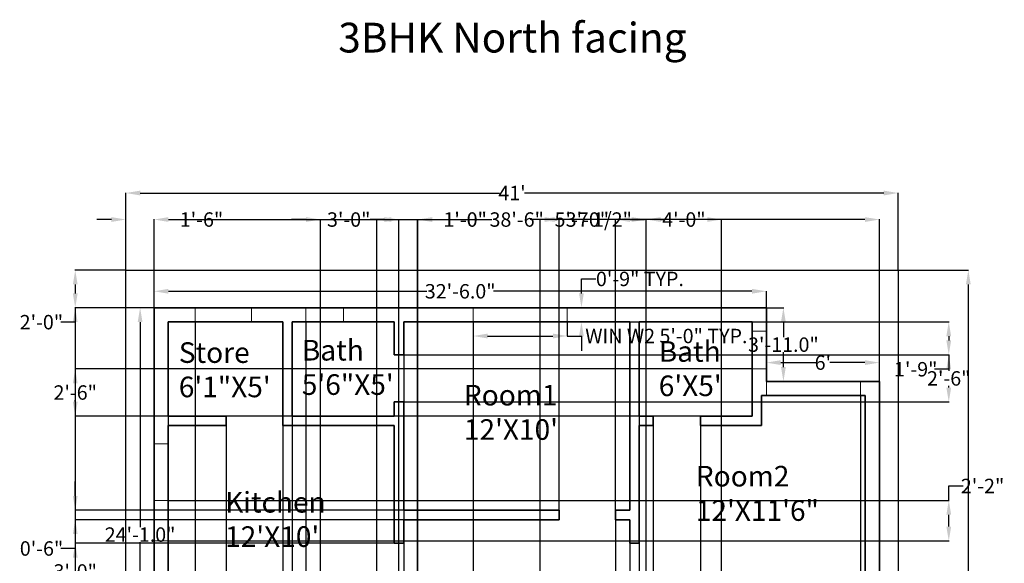
# Model space of a CAD drawing. Units: inches. Extents: x -69 to 558, y -494 to 191.
# Tile 3 of 3: x -69 to 558, y -155 to 191. Entities that reach past the tile are written whole.
import ezdxf

# ---------------------------------------------------------------- set-up
doc = ezdxf.new("R2010")
doc.units = ezdxf.units.IN
doc.header["$MEASUREMENT"] = 0
for name, color, linetype, lineweight in [('A-ANNO-DIMS', 2, 'Continuous', 18), ('A-ANNO-TEXT', 7, 'Continuous', 25), ('A-AREA-IDEN', 7, 'Continuous', 18), ('A-GLAZ', 4, 'Continuous', 18), ('A-WALL', 7, 'Continuous', 35), ('C-PROP', 8, 'Continuous', 25)]:
    doc.layers.add(name, color=color, linetype=linetype, lineweight=lineweight)
doc.styles.get("Standard").update_dxf_attribs({"font": 'arial.ttf'})
doc.dimstyles.get("Standard").update_dxf_attribs({"dimtxt": 9.18, "dimasz": 9.18, "dimexe": 0.18, "dimexo": 0.0625, "dimgap": 0.09, "dimtad": 0, "dimtih": 1, "dimtoh": 1, "dimdec": 1, "dimzin": 0, "dimdsep": 46, "dimlunit": 3, "dimtxsty": 'Standard', "dimcen": 9, "dimadec": 0, "dimazin": 0, "dimtfac": 1, "dimtdec": 1, "dimtofl": 0, "dimtmove": 0, "dimatfit": 3, "dimfxl": 1, "dimtolj": 1, "dimtzin": 0, "dimarcsym": 0})

# ---------------------------------------------------------------- blocks, each defined once
blk = doc.blocks.new('*D8')
at = {"layer": 'A-ANNO-DIMS', "color": 0, "lineweight": -2, "transparency": 16777216}
for p, q in [((490.42, 31.7), (535.2, 31.7)), ((535.02, 22.52), (535.02, -203.53)), ((535.02, -439.12), (535.02, -213.08)), ((490.42, -448.3), (535.2, -448.3))]:
    blk.add_line(p, q, dxfattribs=at)
at = {"layer": 'A-ANNO-DIMS', "color": 0, "transparency": 16777216}
for points in [[(533.49, 22.52), (536.55, 22.52), (535.02, 31.7)], [(533.49, -439.12), (536.55, -439.12), (535.02, -448.3)]]:
    blk.add_solid(points, dxfattribs=at)
at = {"layer": 'Defpoints', "color": 0, "transparency": 16777216}
for p in [(490.36, 31.7), (490.36, -448.3), (535.02, -448.3)]:
    blk.add_point(p, dxfattribs=at)
at = {"layer": 'A-ANNO-DIMS', "color": 0, "transparency": 16777216, "insert": (535.02, -208.3), "char_height": 9.18, "attachment_point": 5}
blk.add_mtext("\\A1;40'", dxfattribs=at)
blk = doc.blocks.new('*D9')
at = {"layer": 'A-ANNO-DIMS', "color": 0, "lineweight": -2, "transparency": 16777216}
for p, q in [((-1.64, 31.76), (-1.64, 80.97)), ((7.54, 80.79), (236.29, 80.79)), ((481.18, 80.79), (252.42, 80.79)), ((490.36, 31.76), (490.36, 80.97))]:
    blk.add_line(p, q, dxfattribs=at)
at = {"layer": 'A-ANNO-DIMS', "color": 0, "transparency": 16777216}
for points in [[(7.54, 82.32), (7.54, 79.26), (-1.64, 80.79)], [(481.18, 82.32), (481.18, 79.26), (490.36, 80.79)]]:
    blk.add_solid(points, dxfattribs=at)
at = {"layer": 'Defpoints', "color": 0, "transparency": 16777216}
for p in [(490.36, 80.79), (-1.64, 31.7), (490.36, 31.7)]:
    blk.add_point(p, dxfattribs=at)
at = {"layer": 'A-ANNO-DIMS', "color": 0, "transparency": 16777216, "insert": (244.36, 80.79), "char_height": 9.18, "attachment_point": 5}
blk.add_mtext("\\A1;41'", dxfattribs=at)
blk = doc.blocks.new('*D10')
at = {"layer": 'A-ANNO-DIMS', "color": 0, "lineweight": -2, "transparency": 16777216}
for p, q in [((16.36, 7.76), (16.36, 18.37)), ((25.54, 18.19), (190.16, 18.19)), ((397.18, 18.19), (232.56, 18.19)), ((406.36, 7.76), (406.36, 18.37))]:
    blk.add_line(p, q, dxfattribs=at)
at = {"layer": 'A-ANNO-DIMS', "color": 0, "transparency": 16777216}
for points in [[(25.54, 19.72), (25.54, 16.66), (16.36, 18.19)], [(397.18, 19.72), (397.18, 16.66), (406.36, 18.19)]]:
    blk.add_solid(points, dxfattribs=at)
at = {"layer": 'Defpoints', "color": 0, "transparency": 16777216}
for p in [(406.36, 18.19), (16.36, 7.7), (406.36, 7.7)]:
    blk.add_point(p, dxfattribs=at)
at = {"layer": 'A-ANNO-DIMS', "color": 0, "transparency": 16777216, "insert": (211.36, 18.19), "char_height": 9.18, "attachment_point": 5}
blk.add_mtext('\\A1;32\'-6.0"', dxfattribs=at)
blk = doc.blocks.new('*D11')
at = {"layer": 'A-ANNO-DIMS', "color": 0, "lineweight": -2, "transparency": 16777216}
for p, q in [((406.36, -39.24), (406.36, -27.06)), ((415.54, -27.24), (438.02, -27.24)), ((469.18, -27.24), (446.7, -27.24)), ((478.36, -39.24), (478.36, -27.06))]:
    blk.add_line(p, q, dxfattribs=at)
at = {"layer": 'A-ANNO-DIMS', "color": 0, "transparency": 16777216}
for points in [[(415.54, -25.71), (415.54, -28.77), (406.36, -27.24)], [(469.18, -25.71), (469.18, -28.77), (478.36, -27.24)]]:
    blk.add_solid(points, dxfattribs=at)
at = {"layer": 'Defpoints', "color": 0, "transparency": 16777216}
for p in [(478.36, -27.24), (406.36, -39.3), (478.36, -39.3)]:
    blk.add_point(p, dxfattribs=at)
at = {"layer": 'A-ANNO-DIMS', "color": 0, "transparency": 16777216, "insert": (442.36, -27.24), "char_height": 9.18, "attachment_point": 5}
blk.add_mtext("\\A1;6'", dxfattribs=at)
blk = doc.blocks.new('*D12')
at = {"layer": 'A-ANNO-DIMS', "color": 0, "lineweight": -2, "transparency": 16777216}
for p, q in [((406.42, 7.7), (417.41, 7.7)), ((417.23, -1.48), (417.23, -11.02)), ((417.23, -30.12), (417.23, -20.59)), ((406.42, -39.3), (417.41, -39.3))]:
    blk.add_line(p, q, dxfattribs=at)
at = {"layer": 'A-ANNO-DIMS', "color": 0, "transparency": 16777216}
for points in [[(415.7, -1.48), (418.76, -1.48), (417.23, 7.7)], [(415.7, -30.12), (418.76, -30.12), (417.23, -39.3)]]:
    blk.add_solid(points, dxfattribs=at)
at = {"layer": 'Defpoints', "color": 0, "transparency": 16777216}
for p in [(406.36, 7.7), (417.23, 7.7), (406.36, -39.3)]:
    blk.add_point(p, dxfattribs=at)
at = {"layer": 'A-ANNO-DIMS', "color": 0, "transparency": 16777216, "insert": (417.23, -15.8), "char_height": 9.18, "attachment_point": 5}
blk.add_mtext('\\A1;3\'-11.0"', dxfattribs=at)
blk = doc.blocks.new('*D13')
at = {"layer": 'A-ANNO-DIMS', "color": 0, "lineweight": -2, "transparency": 16777216}
for p, q in [((16.29, 7.7), (7.29, 7.7)), ((7.47, -1.48), (7.47, -132.03)), ((7.47, -272.12), (7.47, -141.58)), ((16.29, -281.3), (7.29, -281.3))]:
    blk.add_line(p, q, dxfattribs=at)
at = {"layer": 'A-ANNO-DIMS', "color": 0, "transparency": 16777216}
for points in [[(5.94, -1.48), (9, -1.48), (7.47, 7.7)], [(5.94, -272.12), (9, -272.12), (7.47, -281.3)]]:
    blk.add_solid(points, dxfattribs=at)
at = {"layer": 'Defpoints', "color": 0, "transparency": 16777216}
for p in [(7.47, 7.7), (16.36, 7.7), (16.36, -281.3)]:
    blk.add_point(p, dxfattribs=at)
at = {"layer": 'A-ANNO-DIMS', "color": 0, "transparency": 16777216, "insert": (7.47, -136.8), "char_height": 9.18, "attachment_point": 5}
blk.add_mtext('\\A1;24\'-1.0"', dxfattribs=at)
blk = doc.blocks.new('WIN-36IN')
blk.add_lwpolyline([(0, 0), (0, 9), (36, 9), (36, 0)], close=True)
blk = doc.blocks.new('WIN-60IN')
blk.add_lwpolyline([(60, 9), (60, 0), (0, 0), (0, 9)], close=True)
blk = doc.blocks.new('WIN-24IN')
blk.add_lwpolyline([(0, 0), (0, 9), (24, 9), (24, 0)], close=True)
blk = doc.blocks.new('*D20')
at = {"layer": 'A-ANNO-DIMS', "color": 0, "lineweight": -2, "transparency": 16777216}
for p, q in [((219.59, -1.37), (219.59, -10.48)), ((279.59, -1.37), (279.59, -10.48)), ((228.77, -10.3), (270.41, -10.3)), ((279.59, -10.3), (288.77, -10.3))]:
    blk.add_line(p, q, dxfattribs=at)
at = {"layer": 'A-ANNO-DIMS', "color": 0, "transparency": 16777216}
for points in [[(228.77, -8.77), (228.77, -11.83), (219.59, -10.3)], [(270.41, -8.77), (270.41, -11.83), (279.59, -10.3)]]:
    blk.add_solid(points, dxfattribs=at)
at = {"layer": 'Defpoints', "color": 0, "transparency": 16777216}
for p in [(219.59, -1.3), (279.59, -1.3), (279.59, -10.3)]:
    blk.add_point(p, dxfattribs=at)
at = {"layer": 'A-ANNO-DIMS', "color": 0, "transparency": 16777216, "insert": (342.67, -10.3), "char_height": 9.18, "attachment_point": 5}
blk.add_mtext('\\A1;WIN W2 5\'-0" TYP.', dxfattribs=at)
blk = doc.blocks.new('*D21')
at = {"layer": 'A-ANNO-DIMS', "color": 0, "lineweight": -2, "transparency": 16777216}
for p, q in [((288.59, 16.88), (288.59, 26.06)), ((288.59, 26.06), (297.77, 26.06)), ((279.66, 7.7), (288.77, 7.7)), ((279.66, -1.3), (288.77, -1.3)), ((288.59, -10.48), (288.59, -19.66))]:
    blk.add_line(p, q, dxfattribs=at)
at = {"layer": 'A-ANNO-DIMS', "color": 0, "transparency": 16777216}
for points in [[(287.06, 16.88), (290.12, 16.88), (288.59, 7.7)], [(287.06, -10.48), (290.12, -10.48), (288.59, -1.3)]]:
    blk.add_solid(points, dxfattribs=at)
at = {"layer": 'Defpoints', "color": 0, "transparency": 16777216}
for p in [(279.59, 7.7), (288.59, 7.7), (279.59, -1.3)]:
    blk.add_point(p, dxfattribs=at)
at = {"layer": 'A-ANNO-DIMS', "color": 0, "transparency": 16777216, "insert": (325.84, 26.06), "char_height": 9.18, "attachment_point": 5}
blk.add_mtext('\\A1;0\'-9" TYP.', dxfattribs=at)
blk = doc.blocks.new('*D24')
at = {"layer": 'A-ANNO-DIMS', "color": 0, "lineweight": -2, "transparency": 16777216}
for p, q in [((16.36, 7.76), (16.36, 64.08)), ((25.54, 63.9), (231.5, 63.9)), ((469.18, 63.9), (263.21, 63.9)), ((478.36, -39.24), (478.36, 64.08))]:
    blk.add_line(p, q, dxfattribs=at)
at = {"layer": 'A-ANNO-DIMS', "color": 0, "transparency": 16777216}
for points in [[(25.54, 65.43), (25.54, 62.37), (16.36, 63.9)], [(469.18, 65.43), (469.18, 62.37), (478.36, 63.9)]]:
    blk.add_solid(points, dxfattribs=at)
at = {"layer": 'Defpoints', "color": 0, "transparency": 16777216}
for p in [(478.36, 63.9), (16.36, 7.7), (478.36, -39.3)]:
    blk.add_point(p, dxfattribs=at)
at = {"layer": 'A-ANNO-DIMS', "color": 0, "transparency": 16777216, "insert": (247.36, 63.9), "char_height": 9.18, "attachment_point": 5}
blk.add_mtext('\\A1;38\'-6"', dxfattribs=at)
blk = doc.blocks.new('*D25')
at = {"layer": 'A-ANNO-DIMS', "color": 0, "lineweight": -2, "transparency": 16777216}
for p, q in [((16.29, 7.7), (-34.02, 7.7)), ((-33.84, -1.48), (-33.84, -203.52)), ((-33.84, -415.12), (-33.84, -213.09)), ((172.29, -424.3), (-34.02, -424.3))]:
    blk.add_line(p, q, dxfattribs=at)
at = {"layer": 'A-ANNO-DIMS', "color": 0, "transparency": 16777216}
for points in [[(-35.37, -1.48), (-32.31, -1.48), (-33.84, 7.7)], [(-35.37, -415.12), (-32.31, -415.12), (-33.84, -424.3)]]:
    blk.add_solid(points, dxfattribs=at)
at = {"layer": 'Defpoints', "color": 0, "transparency": 16777216}
for p in [(16.36, 7.7), (-33.84, -424.3), (172.36, -424.3)]:
    blk.add_point(p, dxfattribs=at)
at = {"layer": 'A-ANNO-DIMS', "color": 0, "transparency": 16777216, "insert": (-33.84, -208.3), "char_height": 9.18, "attachment_point": 5}
blk.add_mtext('\\A1;36\'-0"', dxfattribs=at)
blk = doc.blocks.new('*D26')
at = {"layer": 'A-ANNO-DIMS', "color": 0, "lineweight": -2, "transparency": 16777216}
for p, q in [((-10.82, 63.9), (-20, 63.9)), ((-1.64, 31.76), (-1.64, 64.08)), ((16.36, 7.76), (16.36, 64.08)), ((25.54, 63.9), (34.72, 63.9))]:
    blk.add_line(p, q, dxfattribs=at)
at = {"layer": 'A-ANNO-DIMS', "color": 0, "transparency": 16777216}
for points in [[(-10.82, 65.43), (-10.82, 62.37), (-1.64, 63.9)], [(25.54, 65.43), (25.54, 62.37), (16.36, 63.9)]]:
    blk.add_solid(points, dxfattribs=at)
at = {"layer": 'Defpoints', "color": 0, "transparency": 16777216}
for p in [(16.36, 63.9), (-1.64, 31.7), (16.36, 7.7)]:
    blk.add_point(p, dxfattribs=at)
at = {"layer": 'A-ANNO-DIMS', "color": 0, "transparency": 16777216, "insert": (46.58, 63.9), "char_height": 9.18, "attachment_point": 5}
blk.add_mtext('\\A1;1\'-6"', dxfattribs=at)
blk = doc.blocks.new('*D27')
at = {"layer": 'A-ANNO-DIMS', "color": 0, "lineweight": -2, "transparency": 16777216}
for p, q in [((-1.71, 31.7), (-34.02, 31.7)), ((-33.84, 22.52), (-33.84, 16.88)), ((16.29, 7.7), (-34.02, 7.7)), ((-33.84, 7.7), (-33.84, -1.48)), ((-33.84, -1.48), (-43.02, -1.48))]:
    blk.add_line(p, q, dxfattribs=at)
at = {"layer": 'A-ANNO-DIMS', "color": 0, "transparency": 16777216}
for points in [[(-35.37, 22.52), (-32.31, 22.52), (-33.84, 31.7)], [(-35.37, 16.88), (-32.31, 16.88), (-33.84, 7.7)]]:
    blk.add_solid(points, dxfattribs=at)
at = {"layer": 'Defpoints', "color": 0, "transparency": 16777216}
for p in [(-1.64, 31.7), (-33.84, 7.7), (16.36, 7.7)]:
    blk.add_point(p, dxfattribs=at)
at = {"layer": 'A-ANNO-DIMS', "color": 0, "transparency": 16777216, "insert": (-55.39, -1.48), "char_height": 9.18, "attachment_point": 5}
blk.add_mtext('\\A1;2\'-0"', dxfattribs=at)
blk = doc.blocks.new('*D30')
at = {"layer": 'A-ANNO-DIMS', "color": 0, "lineweight": -2, "transparency": 16777216}
for p, q in [((113.177437, 63.89515), (103.997437, 63.89515)), ((122.357437, -267.24235), (122.357437, 64.07515)), ((158.357437, -267.24235), (158.357437, 64.07515)), ((167.537437, 63.89515), (176.717437, 63.89515))]:
    blk.add_line(p, q, dxfattribs=at)
at = {"layer": 'A-ANNO-DIMS', "color": 0, "transparency": 16777216}
for points in [[(113.177437, 65.42515), (113.177437, 62.36515), (122.357437, 63.89515)], [(167.537437, 65.42515), (167.537437, 62.36515), (158.357437, 63.89515)]]:
    blk.add_solid(points, dxfattribs=at)
at = {"layer": 'Defpoints', "color": 0, "transparency": 16777216}
for p in [(158.357437, 63.89515), (122.357437, -267.30485), (158.357437, -267.30485)]:
    blk.add_point(p, dxfattribs=at)
at = {"layer": 'A-ANNO-DIMS', "color": 0, "transparency": 16777216, "insert": (140.357437, 63.89515), "char_height": 9.18, "attachment_point": 5}
blk.add_mtext('\\A1;3\'-0"', dxfattribs=at)
blk = doc.blocks.new('*D32')
at = {"layer": 'A-ANNO-DIMS', "color": 0, "lineweight": -2, "transparency": 16777216}
for p, q in [((163.09, 63.9), (153.91, 63.9)), ((172.27, -311.24), (172.27, 64.08)), ((184.27, -311.24), (184.27, 64.08)), ((193.45, 63.9), (202.63, 63.9))]:
    blk.add_line(p, q, dxfattribs=at)
at = {"layer": 'A-ANNO-DIMS', "color": 0, "transparency": 16777216}
for points in [[(163.09, 65.43), (163.09, 62.37), (172.27, 63.9)], [(193.45, 65.43), (193.45, 62.37), (184.27, 63.9)]]:
    blk.add_solid(points, dxfattribs=at)
at = {"layer": 'Defpoints', "color": 0, "transparency": 16777216}
for p in [(184.27, 63.9), (172.27, -311.3), (184.27, -311.3)]:
    blk.add_point(p, dxfattribs=at)
at = {"layer": 'A-ANNO-DIMS', "color": 0, "transparency": 16777216, "insert": (214.49, 63.9), "char_height": 9.18, "attachment_point": 5}
blk.add_mtext('\\A1;1\'-0"', dxfattribs=at)
blk = doc.blocks.new('*D33')
at = {"layer": 'A-ANNO-DIMS', "color": 0, "lineweight": -2, "transparency": 16777216}
for p, q in [((329.86, -415.24), (329.86, 64.08)), ((339.04, 63.9), (341.38, 63.9)), ((368.68, 63.9), (366.33, 63.9)), ((377.86, -415.24), (377.86, 64.08))]:
    blk.add_line(p, q, dxfattribs=at)
at = {"layer": 'A-ANNO-DIMS', "color": 0, "transparency": 16777216}
for points in [[(339.04, 65.43), (339.04, 62.37), (329.86, 63.9)], [(368.68, 65.43), (368.68, 62.37), (377.86, 63.9)]]:
    blk.add_solid(points, dxfattribs=at)
at = {"layer": 'Defpoints', "color": 0, "transparency": 16777216}
for p in [(377.86, 63.9), (329.86, -415.3), (377.86, -415.3)]:
    blk.add_point(p, dxfattribs=at)
at = {"layer": 'A-ANNO-DIMS', "color": 0, "transparency": 16777216, "insert": (353.86, 63.9), "char_height": 9.18, "attachment_point": 5}
blk.add_mtext('\\A1;4\'-0"', dxfattribs=at)
blk = doc.blocks.new('*D34')
at = {"layer": 'A-ANNO-DIMS', "color": 0, "lineweight": -2, "transparency": 16777216}
for p, q in [((265.177437, 63.89515), (255.997437, 63.89515)), ((274.357437, -121.24235), (274.357437, 64.07515)), ((310.357437, -121.24235), (310.357437, 64.07515)), ((319.537437, 63.89515), (328.717437, 63.89515))]:
    blk.add_line(p, q, dxfattribs=at)
at = {"layer": 'A-ANNO-DIMS', "color": 0, "transparency": 16777216}
for points in [[(265.177437, 65.42515), (265.177437, 62.36515), (274.357437, 63.89515)], [(319.537437, 65.42515), (319.537437, 62.36515), (310.357437, 63.89515)]]:
    blk.add_solid(points, dxfattribs=at)
at = {"layer": 'Defpoints', "color": 0, "transparency": 16777216}
for p in [(310.357437, 63.89515), (274.357437, -121.30485), (310.357437, -121.30485)]:
    blk.add_point(p, dxfattribs=at)
at = {"layer": 'A-ANNO-DIMS', "color": 0, "transparency": 16777216, "insert": (292.357437, 63.89515), "char_height": 9.18, "attachment_point": 5}
blk.add_mtext('\\A1;3\'-0"', dxfattribs=at)
blk = doc.blocks.new('*D35')
at = {"layer": 'A-ANNO-DIMS', "color": 0, "lineweight": -2, "transparency": 16777216}
for p, q in [((334.357437, -67.36735), (334.357437, -480.68485)), ((364.357437, -67.36735), (364.357437, -480.68485)), ((325.177437, -480.50485), (315.997437, -480.50485)), ((373.537437, -480.50485), (382.717437, -480.50485))]:
    blk.add_line(p, q, dxfattribs=at)
at = {"layer": 'A-ANNO-DIMS', "color": 0, "transparency": 16777216}
for points in [[(325.177437, -478.97485), (325.177437, -482.03485), (334.357437, -480.50485)], [(373.537437, -478.97485), (373.537437, -482.03485), (364.357437, -480.50485)]]:
    blk.add_solid(points, dxfattribs=at)
at = {"layer": 'Defpoints', "color": 0, "transparency": 16777216}
for p in [(334.357437, -67.30485), (364.357437, -67.30485), (364.357437, -480.50485)]:
    blk.add_point(p, dxfattribs=at)
at = {"layer": 'A-ANNO-DIMS', "color": 0, "transparency": 16777216, "insert": (349.357437, -480.50485), "char_height": 9.18, "attachment_point": 5}
blk.add_mtext('\\A1;2\'-6"', dxfattribs=at)
blk = doc.blocks.new('*D36')
at = {"layer": 'A-ANNO-DIMS', "color": 0, "lineweight": -2, "transparency": 16777216}
for p, q in [((-33.84, -112.12), (-33.84, -102.94)), ((274.29, -121.3), (-34.02, -121.3)), ((274.29, -127.3), (-34.02, -127.3)), ((-33.84, -136.48), (-33.84, -145.66)), ((-33.84, -145.66), (-43.02, -145.66))]:
    blk.add_line(p, q, dxfattribs=at)
at = {"layer": 'A-ANNO-DIMS', "color": 0, "transparency": 16777216}
for points in [[(-35.37, -112.12), (-32.31, -112.12), (-33.84, -121.3)], [(-35.37, -136.48), (-32.31, -136.48), (-33.84, -127.3)]]:
    blk.add_solid(points, dxfattribs=at)
at = {"layer": 'Defpoints', "color": 0, "transparency": 16777216}
for p in [(274.36, -121.3), (-33.84, -127.3), (274.36, -127.3)]:
    blk.add_point(p, dxfattribs=at)
at = {"layer": 'A-ANNO-DIMS', "color": 0, "transparency": 16777216, "insert": (-55.31, -145.66), "char_height": 9.18, "attachment_point": 5}
blk.add_mtext('\\A1;0\'-6"', dxfattribs=at)
blk = doc.blocks.new('*D37')
at = {"layer": 'A-ANNO-DIMS', "color": 0, "lineweight": -2, "transparency": 16777216}
for p, q in [((175.36, -1.37), (175.36, -480.68)), ((219.59, -1.37), (219.59, -480.68)), ((184.54, -480.5), (185.19, -480.5)), ((210.41, -480.5), (209.76, -480.5))]:
    blk.add_line(p, q, dxfattribs=at)
at = {"layer": 'A-ANNO-DIMS', "color": 0, "transparency": 16777216}
for points in [[(184.54, -478.97), (184.54, -482.03), (175.36, -480.5)], [(210.41, -478.97), (210.41, -482.03), (219.59, -480.5)]]:
    blk.add_solid(points, dxfattribs=at)
at = {"layer": 'Defpoints', "color": 0, "transparency": 16777216}
for p in [(175.36, -1.3), (219.59, -1.3), (219.59, -480.5)]:
    blk.add_point(p, dxfattribs=at)
at = {"layer": 'A-ANNO-DIMS', "color": 0, "transparency": 16777216, "insert": (197.48, -480.5), "char_height": 9.18, "attachment_point": 5}
blk.add_mtext('\\A1;3\'-8"', dxfattribs=at)
blk = doc.blocks.new('*D40')
at = {"layer": 'A-ANNO-DIMS', "color": 0, "lineweight": -2, "transparency": 16777216}
for p, q in [((25.36, -1.37), (25.36, -480.68)), ((42.48, -1.37), (42.48, -480.68)), ((16.18, -480.5), (7, -480.5)), ((51.66, -480.5), (60.84, -480.5))]:
    blk.add_line(p, q, dxfattribs=at)
at = {"layer": 'A-ANNO-DIMS', "color": 0, "transparency": 16777216}
for points in [[(16.18, -478.97), (16.18, -482.03), (25.36, -480.5)], [(51.66, -478.97), (51.66, -482.03), (42.48, -480.5)]]:
    blk.add_solid(points, dxfattribs=at)
at = {"layer": 'Defpoints', "color": 0, "transparency": 16777216}
for p in [(25.36, -1.3), (42.48, -1.3), (42.48, -480.5)]:
    blk.add_point(p, dxfattribs=at)
at = {"layer": 'A-ANNO-DIMS', "color": 0, "transparency": 16777216, "insert": (72.7, -480.5), "char_height": 9.18, "attachment_point": 5}
blk.add_mtext('\\A1;1\'-5"', dxfattribs=at)
blk = doc.blocks.new('*D41')
at = {"layer": 'A-ANNO-DIMS', "color": 0, "lineweight": -2, "transparency": 16777216}
for p, q in [((104.36, -1.37), (104.36, -480.68)), ((113.07, -1.37), (113.07, -480.68)), ((95.18, -480.5), (86, -480.5)), ((122.25, -480.5), (131.43, -480.5))]:
    blk.add_line(p, q, dxfattribs=at)
at = {"layer": 'A-ANNO-DIMS', "color": 0, "transparency": 16777216}
for points in [[(95.18, -478.97), (95.18, -482.03), (104.36, -480.5)], [(122.25, -478.97), (122.25, -482.03), (113.07, -480.5)]]:
    blk.add_solid(points, dxfattribs=at)
at = {"layer": 'Defpoints', "color": 0, "transparency": 16777216}
for p in [(104.36, -1.3), (113.07, -1.3), (113.07, -480.5)]:
    blk.add_point(p, dxfattribs=at)
at = {"layer": 'A-ANNO-DIMS', "color": 0, "transparency": 16777216, "insert": (154.42, -480.5), "char_height": 9.18, "attachment_point": 5}
blk.add_mtext('\\A1;0\'-8 1/2"', dxfattribs=at)
blk = doc.blocks.new('*D42')
at = {"layer": 'A-ANNO-DIMS', "color": 0, "lineweight": -2, "transparency": 16777216}
for p, q in [((397.29, -31.3), (-34.02, -31.3)), ((-33.84, -40.48), (-33.84, -41.53)), ((-33.84, -52.12), (-33.84, -51.08)), ((397.29, -61.3), (-34.02, -61.3))]:
    blk.add_line(p, q, dxfattribs=at)
at = {"layer": 'A-ANNO-DIMS', "color": 0, "transparency": 16777216}
for points in [[(-35.37, -40.48), (-32.31, -40.48), (-33.84, -31.3)], [(-35.37, -52.12), (-32.31, -52.12), (-33.84, -61.3)]]:
    blk.add_solid(points, dxfattribs=at)
at = {"layer": 'Defpoints', "color": 0, "transparency": 16777216}
for p in [(397.36, -31.3), (-33.84, -61.3), (397.36, -61.3)]:
    blk.add_point(p, dxfattribs=at)
at = {"layer": 'A-ANNO-DIMS', "color": 0, "transparency": 16777216, "insert": (-33.84, -46.3), "char_height": 9.18, "attachment_point": 5}
blk.add_mtext('\\A1;2\'-6"', dxfattribs=at)
blk = doc.blocks.new('*D43')
at = {"layer": 'A-ANNO-DIMS', "color": 0, "lineweight": -2, "transparency": 16777216}
for p, q in [((466.36, -48.37), (466.36, -480.68)), ((469.36, -48.37), (469.36, -480.68)), ((457.18, -480.5), (448, -480.5)), ((478.54, -480.5), (487.72, -480.5))]:
    blk.add_line(p, q, dxfattribs=at)
at = {"layer": 'A-ANNO-DIMS', "color": 0, "transparency": 16777216}
for points in [[(457.18, -478.97), (457.18, -482.03), (466.36, -480.5)], [(478.54, -478.97), (478.54, -482.03), (469.36, -480.5)]]:
    blk.add_solid(points, dxfattribs=at)
at = {"layer": 'Defpoints', "color": 0, "transparency": 16777216}
for p in [(466.36, -48.3), (469.36, -48.3), (469.36, -480.5)]:
    blk.add_point(p, dxfattribs=at)
at = {"layer": 'A-ANNO-DIMS', "color": 0, "transparency": 16777216, "insert": (500.01, -480.5), "char_height": 9.18, "attachment_point": 5}
blk.add_mtext('\\A1;0\'-3"', dxfattribs=at)
blk = doc.blocks.new('*D45')
at = {"layer": 'A-ANNO-DIMS', "color": 0, "lineweight": -2, "transparency": 16777216}
for p, q in [((522.56, -115.02), (522.56, -105.84)), ((522.56, -105.84), (531.74, -105.84)), ((25.42, -115.02), (522.74, -115.02)), ((522.56, -131.69), (522.56, -124.2)), ((25.42, -140.87), (522.74, -140.87))]:
    blk.add_line(p, q, dxfattribs=at)
at = {"layer": 'A-ANNO-DIMS', "color": 0, "transparency": 16777216}
for points in [[(521.03, -124.2), (524.09, -124.2), (522.56, -115.02)], [(521.03, -131.69), (524.09, -131.69), (522.56, -140.87)]]:
    blk.add_solid(points, dxfattribs=at)
at = {"layer": 'Defpoints', "color": 0, "transparency": 16777216}
for p in [(25.36, -115.02), (522.56, -115.02), (25.36, -140.87)]:
    blk.add_point(p, dxfattribs=at)
at = {"layer": 'A-ANNO-DIMS', "color": 0, "transparency": 16777216, "insert": (544.11, -105.84), "char_height": 9.18, "attachment_point": 5}
blk.add_mtext('\\A1;2\'-2"', dxfattribs=at)
blk = doc.blocks.new('*D47')
at = {"layer": 'A-ANNO-DIMS', "color": 0, "lineweight": -2, "transparency": 16777216}
for p, q in [((262.36, -415.24), (262.36, 64.08)), ((271.54, 63.9), (273.12, 63.9)), ((320.68, 63.9), (319.09, 63.9)), ((329.86, -415.24), (329.86, 64.08))]:
    blk.add_line(p, q, dxfattribs=at)
at = {"layer": 'A-ANNO-DIMS', "color": 0, "transparency": 16777216}
for points in [[(271.54, 65.43), (271.54, 62.37), (262.36, 63.9)], [(320.68, 65.43), (320.68, 62.37), (329.86, 63.9)]]:
    blk.add_solid(points, dxfattribs=at)
at = {"layer": 'Defpoints', "color": 0, "transparency": 16777216}
for p in [(329.86, 63.9), (262.36, -415.3), (329.86, -415.3)]:
    blk.add_point(p, dxfattribs=at)
at = {"layer": 'A-ANNO-DIMS', "color": 0, "transparency": 16777216, "insert": (296.11, 63.9), "char_height": 9.18, "attachment_point": 5}
blk.add_mtext('\\A1;5\'-7 1/2"', dxfattribs=at)
blk = doc.blocks.new('*D48')
at = {"layer": 'A-ANNO-DIMS', "color": 0, "lineweight": -2, "transparency": 16777216}
for p, q in [((310.36, -127.37), (310.36, -480.68)), ((319.36, -127.37), (319.36, -480.68)), ((301.18, -480.5), (292, -480.5)), ((328.54, -480.5), (337.72, -480.5))]:
    blk.add_line(p, q, dxfattribs=at)
at = {"layer": 'A-ANNO-DIMS', "color": 0, "transparency": 16777216}
for points in [[(301.18, -478.97), (301.18, -482.03), (310.36, -480.5)], [(328.54, -478.97), (328.54, -482.03), (319.36, -480.5)]]:
    blk.add_solid(points, dxfattribs=at)
at = {"layer": 'Defpoints', "color": 0, "transparency": 16777216}
for p in [(310.36, -127.3), (319.36, -127.3), (319.36, -480.5)]:
    blk.add_point(p, dxfattribs=at)
at = {"layer": 'A-ANNO-DIMS', "color": 0, "transparency": 16777216, "insert": (350.01, -480.5), "char_height": 9.18, "attachment_point": 5}
blk.add_mtext('\\A1;0\'-9"', dxfattribs=at)
blk = doc.blocks.new('*D49')
at = {"layer": 'A-ANNO-DIMS', "color": 0, "lineweight": -2, "transparency": 16777216}
for p, q in [((325.36, -61.37), (325.36, -480.68)), ((334.36, -61.37), (334.36, -480.68)), ((316.18, -480.5), (307, -480.5)), ((343.54, -480.5), (352.72, -480.5))]:
    blk.add_line(p, q, dxfattribs=at)
at = {"layer": 'A-ANNO-DIMS', "color": 0, "transparency": 16777216}
for points in [[(316.18, -478.97), (316.18, -482.03), (325.36, -480.5)], [(343.54, -478.97), (343.54, -482.03), (334.36, -480.5)]]:
    blk.add_solid(points, dxfattribs=at)
at = {"layer": 'Defpoints', "color": 0, "transparency": 16777216}
for p in [(325.36, -61.3), (334.36, -61.3), (334.36, -480.5)]:
    blk.add_point(p, dxfattribs=at)
at = {"layer": 'A-ANNO-DIMS', "color": 0, "transparency": 16777216, "insert": (365.01, -480.5), "char_height": 9.18, "attachment_point": 5}
blk.add_mtext('\\A1;0\'-9"', dxfattribs=at)
blk = doc.blocks.new('*D50')
at = {"layer": 'A-ANNO-DIMS', "color": 0, "lineweight": -2, "transparency": 16777216}
for p, q in [((169.29, -142.3), (-34.02, -142.3)), ((-33.84, -151.48), (-33.84, -155.52)), ((-33.84, -169.12), (-33.84, -165.09)), ((169.29, -178.3), (-34.02, -178.3))]:
    blk.add_line(p, q, dxfattribs=at)
at = {"layer": 'A-ANNO-DIMS', "color": 0, "transparency": 16777216}
for points in [[(-35.37, -151.48), (-32.31, -151.48), (-33.84, -142.3)], [(-35.37, -169.12), (-32.31, -169.12), (-33.84, -178.3)]]:
    blk.add_solid(points, dxfattribs=at)
at = {"layer": 'Defpoints', "color": 0, "transparency": 16777216}
for p in [(169.36, -142.3), (-33.84, -178.3), (169.36, -178.3)]:
    blk.add_point(p, dxfattribs=at)
at = {"layer": 'A-ANNO-DIMS', "color": 0, "transparency": 16777216, "insert": (-33.84, -160.3), "char_height": 9.18, "attachment_point": 5}
blk.add_mtext('\\A1;3\'-0"', dxfattribs=at)
blk = doc.blocks.new('*D56')
at = {"layer": 'A-ANNO-DIMS', "color": 0, "lineweight": -2, "transparency": 16777216}
for p, q in [((62.357437, -67.36735), (62.357437, -480.68485)), ((98.357437, -67.36735), (98.357437, -480.68485)), ((53.177437, -480.50485), (43.997437, -480.50485)), ((107.537437, -480.50485), (116.717437, -480.50485))]:
    blk.add_line(p, q, dxfattribs=at)
at = {"layer": 'A-ANNO-DIMS', "color": 0, "transparency": 16777216}
for points in [[(53.177437, -478.97485), (53.177437, -482.03485), (62.357437, -480.50485)], [(107.537437, -478.97485), (107.537437, -482.03485), (98.357437, -480.50485)]]:
    blk.add_solid(points, dxfattribs=at)
at = {"layer": 'Defpoints', "color": 0, "transparency": 16777216}
for p in [(62.357437, -67.30485), (98.357437, -67.30485), (98.357437, -480.50485)]:
    blk.add_point(p, dxfattribs=at)
at = {"layer": 'A-ANNO-DIMS', "color": 0, "transparency": 16777216, "insert": (80.357437, -480.50485), "char_height": 9.18, "attachment_point": 5}
blk.add_mtext('\\A1;3\'-0"', dxfattribs=at)
blk = doc.blocks.new('*D57')
at = {"layer": 'A-ANNO-DIMS', "color": 0, "lineweight": -2, "transparency": 16777216}
for p, q in [((175.42, -22.3), (522.74, -22.3)), ((522.56, -31.48), (522.56, -32.53)), ((522.56, -43.12), (522.56, -42.08)), ((175.42, -52.3), (522.74, -52.3))]:
    blk.add_line(p, q, dxfattribs=at)
at = {"layer": 'A-ANNO-DIMS', "color": 0, "transparency": 16777216}
for points in [[(521.03, -31.48), (524.09, -31.48), (522.56, -22.3)], [(521.03, -43.12), (524.09, -43.12), (522.56, -52.3)]]:
    blk.add_solid(points, dxfattribs=at)
at = {"layer": 'Defpoints', "color": 0, "transparency": 16777216}
for p in [(175.36, -22.3), (175.36, -52.3), (522.56, -52.3)]:
    blk.add_point(p, dxfattribs=at)
at = {"layer": 'A-ANNO-DIMS', "color": 0, "transparency": 16777216, "insert": (522.56, -37.3), "char_height": 9.18, "attachment_point": 5}
blk.add_mtext('\\A1;2\'-6"', dxfattribs=at)
blk = doc.blocks.new('*D58')
at = {"layer": 'A-ANNO-DIMS', "color": 0, "lineweight": -2, "transparency": 16777216}
for p, q in [((175.42, -1.3), (522.74, -1.3)), ((522.56, -10.48), (522.56, -13.12)), ((175.42, -22.3), (522.74, -22.3)), ((522.56, -22.3), (522.56, -31.48)), ((522.56, -31.48), (513.38, -31.48))]:
    blk.add_line(p, q, dxfattribs=at)
at = {"layer": 'A-ANNO-DIMS', "color": 0, "transparency": 16777216}
for points in [[(521.03, -10.48), (524.09, -10.48), (522.56, -1.3)], [(521.03, -13.12), (524.09, -13.12), (522.56, -22.3)]]:
    blk.add_solid(points, dxfattribs=at)
at = {"layer": 'Defpoints', "color": 0, "transparency": 16777216}
for p in [(175.36, -1.3), (175.36, -22.3), (522.56, -22.3)]:
    blk.add_point(p, dxfattribs=at)
at = {"layer": 'A-ANNO-DIMS', "color": 0, "transparency": 16777216, "insert": (501.52, -31.48), "char_height": 9.18, "attachment_point": 5}
blk.add_mtext('\\A1;1\'-9"', dxfattribs=at)
blk = doc.blocks.new('*D61')
at = {"layer": 'A-ANNO-DIMS', "color": 0, "lineweight": -2, "transparency": 16777216}
for p, q in [((163.18, 63.9), (154, 63.9)), ((172.36, -424.24), (172.36, 64.08)), ((184.36, -424.24), (184.36, 64.08)), ((193.54, 63.9), (202.72, 63.9))]:
    blk.add_line(p, q, dxfattribs=at)
at = {"layer": 'A-ANNO-DIMS', "color": 0, "transparency": 16777216}
for points in [[(163.18, 65.43), (163.18, 62.37), (172.36, 63.9)], [(193.54, 65.43), (193.54, 62.37), (184.36, 63.9)]]:
    blk.add_solid(points, dxfattribs=at)
at = {"layer": 'Defpoints', "color": 0, "transparency": 16777216}
for p in [(184.36, 63.9), (172.36, -424.3), (184.36, -424.3)]:
    blk.add_point(p, dxfattribs=at)
at = {"layer": 'A-ANNO-DIMS', "color": 0, "transparency": 16777216, "insert": (214.58, 63.9), "char_height": 9.18, "attachment_point": 5}
blk.add_mtext('\\A1;1\'-0"', dxfattribs=at)

msp = doc.modelspace()

# ---------------------------------------------------------------- linework, layer by layer
at = {"layer": 'A-WALL'}
for p, q in [((16.36, -281.3), (16.36, 7.7)), ((16.36, 7.7), (406.36, 7.7)), ((406.36, -39.3), (406.36, 7.7)), ((25.36, -1.3), (98.36, -1.3)), ((25.36, -61.3), (25.36, -1.3)), ((98.36, -67.3), (98.36, -1.3)), ((104.36, -61.3), (104.36, -1.3)), ((104.36, -1.3), (169.36, -1.3)), ((169.36, -22.3), (169.36, -1.3)), ((175.36, -1.3), (319.36, -1.3)), ((175.36, -22.3), (175.36, -1.3)), ((319.36, -121.3), (319.36, -1.3)), ((325.36, -1.3), (397.36, -1.3)), ((325.36, -61.3), (325.36, -1.3)), ((397.36, -61.3), (397.36, -1.3)), ((169.36, -22.3), (175.36, -22.3)), ((406.36, -39.3), (478.36, -39.3)), ((478.36, -196.3), (478.36, -39.3)), ((403.36, -67.3), (403.36, -48.3)), ((403.36, -48.3), (469.36, -48.3)), ((469.36, -187.3), (469.36, -48.3)), ((169.36, -61.3), (169.36, -52.3)), ((169.36, -52.3), (175.36, -52.3)), ((175.36, -121.3), (175.36, -52.3)), ((25.36, -61.3), (62.36, -61.3)), ((62.36, -67.3), (62.36, -61.3)), ((104.36, -61.3), (169.36, -61.3)), ((325.36, -61.3), (334.36, -61.3)), ((334.36, -67.3), (334.36, -61.3)), ((364.36, -67.3), (364.36, -61.3)), ((364.36, -61.3), (397.36, -61.3)), ((25.36, -67.3), (62.36, -67.3)), ((25.36, -187.3), (25.36, -67.3)), ((98.36, -67.3), (169.36, -67.3)), ((169.36, -142.3), (169.36, -67.3)), ((325.36, -67.3), (334.36, -67.3)), ((325.36, -142.3), (325.36, -67.3)), ((364.36, -67.3), (403.36, -67.3)), ((175.36, -121.3), (274.36, -121.3)), ((274.36, -127.3), (274.36, -121.3)), ((310.36, -127.3), (310.36, -121.3)), ((310.36, -121.3), (319.36, -121.3)), ((175.36, -127.3), (274.36, -127.3)), ((175.36, -142.3), (175.36, -127.3)), ((310.36, -127.3), (319.36, -127.3)), ((319.36, -142.3), (319.36, -127.3)), ((169.36, -142.3), (175.36, -142.3)), ((319.36, -142.3), (325.36, -142.3))]:
    msp.add_line(p, q, dxfattribs=at)
at = {"layer": 'C-PROP'}
for p, q in [((-1.64, 31.7), (490.36, 31.7)), ((-1.64, -448.3), (-1.64, 31.7)), ((490.36, 31.7), (490.36, -448.3))]:
    msp.add_line(p, q, dxfattribs=at)

# ---------------------------------------------------------------- block references
at = {"layer": 'A-GLAZ'}
for name, p in [('WIN-36IN', (42.48, -1.3)), ('WIN-24IN', (113.07, -1.3)), ('WIN-60IN', (219.59, -1.3)), ('WIN-60IN', (406.36, -48.3))]:
    msp.add_blockref(name, p, dxfattribs=at)
for name, p, rotation in [('WIN-24IN', (397.36, -7.3), 269.9999999999997), ('WIN-36IN', (16.36, -79.02), 270), ('WIN-36IN', (16.36, -140.87), 270)]:
    msp.add_blockref(name, p, dxfattribs=dict(at, rotation=rotation))

# ---------------------------------------------------------------- texts
at = {"layer": 'A-ANNO-TEXT', "insert": (133.72, 189.25), "char_height": 18.9464, "attachment_point": 1}
msp.add_mtext_dynamic_manual_height_columns('3BHK North facing ', width=251.9271, gutter_width=94.73, heights=[87.21], dxfattribs=at)
at = {"layer": 'A-AREA-IDEN', "char_height": 13.129, "attachment_point": 1}
for s, insert in [('Bath\\P5\'6"X5\'', (110.48, -12.79)), ("Bath\\P6'X5'", (337.83, -13.57)), ('Store\\P6\'1"X5\'', (32.12, -14.29)), ("Room1\\P12'X10'", (213.68, -41.42)), ('Room2 \\P12\'X11\'6"', (361.43, -93.03)), ("Kitchen\\P12'X10'", (61.6, -109.65))]:
    msp.add_mtext_dynamic_manual_height_columns(s, width=125.4475, gutter_width=65.65, heights=[60.44], dxfattribs=dict(at, insert=insert))

# ---------------------------------------------------------------- dimensions: what is measured, and where the dimension line sits
at = {"layer": 'A-ANNO-DIMS'}
for base, p1, p2, override, picture, middle in [((490.36, 80.79), (-1.64, 31.7), (490.36, 31.7), {"dimclrd": 0, "dimclre": 0, "dimclrt": 0}, '*D9', (244.36, 80.79)), ((329.86, 63.9), (262.36, -415.3), (329.86, -415.3), {"dimdec": 1, "dimlfac": 1, "dimrnd": 0, "dimzin": 1, "dimdsep": 46, "dimlunit": 4, "dimfrac": 2}, '*D47', (296.11, 63.9)), ((16.36, 63.9), (-1.64, 31.7), (16.36, 7.7), {"dimdec": 1, "dimlfac": 1, "dimrnd": 0, "dimzin": 1, "dimdsep": 46, "dimlunit": 4, "dimfrac": 2}, '*D26', (46.58, 63.9)), ((478.36, 63.9), (16.36, 7.7), (478.36, -39.3), {"dimdec": 1, "dimlfac": 1, "dimrnd": 0, "dimzin": 1, "dimdsep": 46, "dimlunit": 4, "dimfrac": 2}, '*D24', (247.36, 63.9)), ((158.36, 63.9), (122.36, -267.3), (158.36, -267.3), {"dimdec": 1, "dimlfac": 1, "dimrnd": 0, "dimzin": 1, "dimdsep": 46, "dimlunit": 4, "dimfrac": 2}, '*D30', (140.36, 63.9)), ((184.27, 63.9), (172.27, -311.3), (184.27, -311.3), {"dimdec": 1, "dimlfac": 1, "dimrnd": 0, "dimzin": 1, "dimdsep": 46, "dimlunit": 4, "dimfrac": 2}, '*D32', (214.49, 63.9)), ((184.36, 63.9), (172.36, -424.3), (184.36, -424.3), {"dimdec": 1, "dimlfac": 1, "dimrnd": 0, "dimzin": 1, "dimdsep": 46, "dimlunit": 4, "dimfrac": 2}, '*D61', (214.58, 63.9)), ((310.36, 63.9), (274.36, -121.3), (310.36, -121.3), {"dimdec": 1, "dimlfac": 1, "dimrnd": 0, "dimzin": 1, "dimdsep": 46, "dimlunit": 4, "dimfrac": 2}, '*D34', (292.36, 63.9)), ((377.86, 63.9), (329.86, -415.3), (377.86, -415.3), {"dimdec": 1, "dimlfac": 1, "dimrnd": 0, "dimzin": 1, "dimdsep": 46, "dimlunit": 4, "dimfrac": 2}, '*D33', (353.86, 63.9)), ((406.36, 18.19), (16.36, 7.7), (406.36, 7.7), {"dimclrd": 0, "dimclre": 0, "dimclrt": 0}, '*D10', (211.36, 18.19)), ((42.48, -480.5), (25.36, -1.3), (42.48, -1.3), {"dimdec": 1, "dimlfac": 1, "dimrnd": 0, "dimzin": 1, "dimdsep": 46, "dimlunit": 4, "dimfrac": 2}, '*D40', (72.7, -480.5)), ((113.07, -480.5), (104.36, -1.3), (113.07, -1.3), {"dimdec": 1, "dimlfac": 1, "dimrnd": 0, "dimzin": 1, "dimdsep": 46, "dimlunit": 4, "dimfrac": 2}, '*D41', (154.42, -480.5)), ((219.59, -480.5), (175.36, -1.3), (219.59, -1.3), {"dimdec": 1, "dimlfac": 1, "dimrnd": 0, "dimzin": 1, "dimdsep": 46, "dimlunit": 4, "dimfrac": 2}, '*D37', (197.48, -480.5)), ((478.36, -27.24), (406.36, -39.3), (478.36, -39.3), {"dimclrd": 0, "dimclre": 0, "dimclrt": 0}, '*D11', (442.36, -27.24)), ((469.36, -480.5), (466.36, -48.3), (469.36, -48.3), {"dimdec": 1, "dimlfac": 1, "dimrnd": 0, "dimzin": 1, "dimdsep": 46, "dimlunit": 4, "dimfrac": 2}, '*D43', (500.01, -480.5)), ((334.36, -480.5), (325.36, -61.3), (334.36, -61.3), {"dimdec": 1, "dimlfac": 1, "dimrnd": 0, "dimzin": 1, "dimdsep": 46, "dimlunit": 4, "dimfrac": 2}, '*D49', (365.01, -480.5)), ((98.36, -480.5), (62.36, -67.3), (98.36, -67.3), {"dimdec": 1, "dimlfac": 1, "dimrnd": 0, "dimzin": 1, "dimdsep": 46, "dimlunit": 4, "dimfrac": 2}, '*D56', (80.36, -480.5)), ((364.36, -480.5), (334.36, -67.3), (364.36, -67.3), {"dimdec": 1, "dimlfac": 1, "dimrnd": 0, "dimzin": 1, "dimdsep": 46, "dimlunit": 4, "dimfrac": 2}, '*D35', (349.36, -480.5)), ((319.36, -480.5), (310.36, -127.3), (319.36, -127.3), {"dimdec": 1, "dimlfac": 1, "dimrnd": 0, "dimzin": 1, "dimdsep": 46, "dimlunit": 4, "dimfrac": 2}, '*D48', (350.01, -480.5))]:
    dim = msp.add_linear_dim(base=base, p1=p1, p2=p2, dimstyle='Standard', override=override, dxfattribs=at)
    dim.commit()
    dim.dimension.update_dxf_attribs({"geometry": picture, "text_midpoint": middle})
dim = msp.add_linear_dim(base=(288.59, 7.7), p1=(279.59, -1.3), p2=(279.59, 7.7), angle=90, text='<> TYP.', dimstyle='Standard', override={"dimdec": 1, "dimlfac": 1, "dimrnd": 0, "dimzin": 1, "dimdsep": 46, "dimlunit": 4, "dimfrac": 2}, dxfattribs=at)
dim.commit()
dim.dimension.update_dxf_attribs({"geometry": '*D21', "text_midpoint": (325.84, 26.06)})
for base, p1, p2, override, picture, middle in [((-33.84, 7.7), (-1.64, 31.7), (16.36, 7.7), {"dimdec": 1, "dimlfac": 1, "dimrnd": 0, "dimzin": 1, "dimdsep": 46, "dimlunit": 4, "dimfrac": 2}, '*D27', (-55.39, -1.48)), ((535.02, -448.3), (490.36, 31.7), (490.36, -448.3), {"dimclrd": 0, "dimclre": 0, "dimclrt": 0}, '*D8', (535.02, -208.3)), ((-33.84, -424.3), (16.36, 7.7), (172.36, -424.3), {"dimdec": 1, "dimlfac": 1, "dimrnd": 0, "dimzin": 1, "dimdsep": 46, "dimlunit": 4, "dimfrac": 2}, '*D25', (-33.84, -208.3)), ((7.47, 7.7), (16.36, -281.3), (16.36, 7.7), {"dimclrd": 0, "dimclre": 0, "dimclrt": 0}, '*D13', (7.47, -136.8)), ((417.23, 7.7), (406.36, -39.3), (406.36, 7.7), {"dimclrd": 0, "dimclre": 0, "dimclrt": 0}, '*D12', (417.23, -15.8)), ((522.56, -22.3), (175.36, -1.3), (175.36, -22.3), {"dimdec": 1, "dimlfac": 1, "dimrnd": 0, "dimzin": 1, "dimdsep": 46, "dimlunit": 4, "dimfrac": 2}, '*D58', (501.52, -31.48)), ((522.56, -52.3), (175.36, -22.3), (175.36, -52.3), {"dimdec": 1, "dimlfac": 1, "dimrnd": 0, "dimzin": 1, "dimdsep": 46, "dimlunit": 4, "dimfrac": 2}, '*D57', (522.56, -37.3)), ((-33.84, -61.3), (397.36, -31.3), (397.36, -61.3), {"dimdec": 1, "dimlfac": 1, "dimrnd": 0, "dimzin": 1, "dimdsep": 46, "dimlunit": 4, "dimfrac": 2}, '*D42', (-33.84, -46.3)), ((522.5574, -115.0186), (25.3574, -140.8735), (25.3574, -115.0186), {"dimdec": 1, "dimlfac": 1, "dimrnd": 0, "dimzin": 1, "dimdsep": 46, "dimlunit": 4, "dimfrac": 2}, '*D45', (544.1071, -105.8386)), ((-33.84, -127.3), (274.36, -121.3), (274.36, -127.3), {"dimdec": 1, "dimlfac": 1, "dimrnd": 0, "dimzin": 1, "dimdsep": 46, "dimlunit": 4, "dimfrac": 2}, '*D36', (-55.31, -145.66)), ((-33.84, -178.3), (169.36, -142.3), (169.36, -178.3), {"dimdec": 1, "dimlfac": 1, "dimrnd": 0, "dimzin": 1, "dimdsep": 46, "dimlunit": 4, "dimfrac": 2}, '*D50', (-33.84, -160.3))]:
    dim = msp.add_linear_dim(base=base, p1=p1, p2=p2, angle=90, dimstyle='Standard', override=override, dxfattribs=at)
    dim.commit()
    dim.dimension.update_dxf_attribs({"geometry": picture, "text_midpoint": middle})
dim = msp.add_linear_dim(base=(279.59, -10.3), p1=(219.59, -1.3), p2=(279.59, -1.3), text='WIN W2 <> TYP.', dimstyle='Standard', override={"dimdec": 1, "dimlfac": 1, "dimrnd": 0, "dimzin": 1, "dimdsep": 46, "dimlunit": 4, "dimfrac": 2}, dxfattribs=at)
dim.commit()
dim.dimension.update_dxf_attribs({"geometry": '*D20', "text_midpoint": (342.67, -10.3)})

doc.saveas('drawing.dxf')
